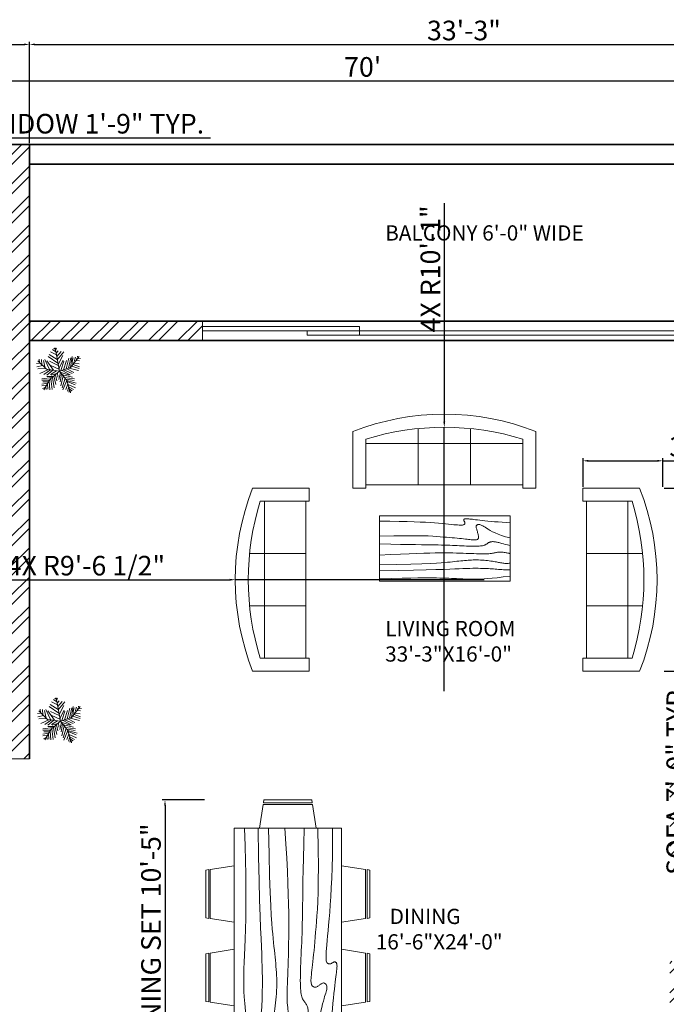
# Model space of a CAD drawing. Units: inches. Extents: x 416 to 1422, y 799 to 1634.
# Tile 3 of 5: x 746 to 1043, y 1174 to 1626. Entities that reach past the tile are written whole.
import ezdxf

# ---------------------------------------------------------------- set-up
doc = ezdxf.new("R2010")
doc.units = ezdxf.units.IN
doc.linetypes.add('ACAD_ISO02W100', pattern=[15, 12, -3])
for name, color, linetype, lineweight in [('A-ANNO-DIMS', 2, 'Continuous', 18), ('A-AREA-IDEN', 7, 'Continuous', 18), ('A-FURN', 8, 'Continuous', 18), ('A-GLAZ', 244, 'Continuous', 18), ('A-WALL', 7, 'Continuous', 35), ('A-WALL-HIDN', 7, 'ACAD_ISO02W100', 18), ('A-WALL-PATT', 252, 'Continuous', 13), ('L-PLNT', 3, 'Continuous', 13)]:
    doc.layers.add(name, color=color, linetype=linetype, lineweight=lineweight)
doc.styles.get("Standard").update_dxf_attribs({"font": 'arial.ttf'})
doc.dimstyles.new('ISO-25', dxfattribs={"dimtxt": 9, "dimasz": 2.5, "dimexe": 1.25, "dimexo": 0.625, "dimtad": 1, "dimlunit": 3, "dimtxsty": 'Standard', "dimcen": 2.5, "dimadec": 0, "dimazin": 0, "dimtfac": 1, "dimtmove": 0, "dimatfit": 3, "dimfxl": 1, "dimarcsym": 0})

# ---------------------------------------------------------------- blocks, each defined once
blk = doc.blocks.new('Dining Set - 36 x 72 in.')
for p, q in [((-22, 27.5), (-22.1562, 26.50042)), ((-5.8416, 26.5), (-22.1534, 26.5)), ((-22, 27.5), (-6, 27.5)), ((-5.8437, 26.49966), (-6, 27.5)), ((6, 27.5), (5.8438, 26.50042)), ((22.1584, 26.5), (5.8466, 26.5)), ((6, 27.5), (22, 27.5)), ((22.1563, 26.49966), (22, 27.5)), ((-22.2343, 26.00059), (-23.4847, 17.99762)), ((-22.2304, 26), (-5.7608, 26)), ((-4.5152, 17.99762), (-5.7655, 25.99926)), ((5.7657, 26.00059), (4.5153, 17.99762)), ((5.7696, 26), (22.2392, 26)), ((23.4848, 17.99762), (22.2345, 25.99926)), ((36, 18), (-36, 18)), ((-36, 18), (-36, -18)), ((36, -18), (36, 18)), ((-45.5, 8), (-44.5004, 8.15617)), ((-45.5, 8), (-45.5, -8)), ((-44.5, -8.15843), (-44.5, 8.15338)), ((-44.0006, 8.23428), (-35.9976, 9.48474)), ((-44, 8.23041), (-44, -8.23915)), ((44.0006, 8.23428), (35.9976, 9.48474)), ((44, 8.23041), (44, -8.23915)), ((44.5, -8.15843), (44.5, 8.15338)), ((45.5, 8), (44.5005, 8.15617)), ((45.5, 8), (45.5, -8)), ((-44.4997, -8.15631), (-45.5, -8)), ((-35.9976, -9.48476), (-43.9993, -8.2345)), ((35.9976, -9.48476), (43.9993, -8.2345)), ((44.4997, -8.15631), (45.5, -8)), ((-36, -18), (36, -18)), ((-22.2343, -26.0006), (-23.4847, -17.99762)), ((-4.5152, -17.99762), (-5.7655, -25.99928)), ((5.7657, -26.0006), (4.5153, -17.99762)), ((23.4848, -17.99762), (22.2345, -25.99928)), ((-22.2304, -26), (-5.7608, -26)), ((5.7696, -26), (22.2392, -26)), ((-22, -27.5), (-22.1562, -26.50044)), ((-5.8416, -26.5), (-22.1534, -26.5)), ((-22, -27.5), (-6, -27.5)), ((-5.8437, -26.49967), (-6, -27.5)), ((6, -27.5), (5.8438, -26.50044)), ((22.1584, -26.5), (5.8466, -26.5)), ((6, -27.5), (22, -27.5)), ((22.1563, -26.49967), (22, -27.5))]:
    blk.add_line(p, q)
for points in [[(-36, 15), (-31.1772, 14.97754), (-26.8079, 14.91406), (-22.8538, 14.81543), (-19.276, 14.6875), (-16.0362, 14.53613), (-13.0957, 14.36718), (-10.4159, 14.18652), (-7.9583, 14), (-5.6904, 13.81315), (-3.6035, 13.63021), (-1.6954, 13.45508), (0.0365, 13.29166), (1.5945, 13.14388), (2.9811, 13.01562), (4.1988, 12.9108), (5.25, 12.83333), (6.1393, 12.78613), (6.8802, 12.76823), (7.4883, 12.77767), (7.9792, 12.8125), (8.3685, 12.87077), (8.6719, 12.95052), (8.9049, 13.0498), (9.0833, 13.16666), (9.2205, 13.29899), (9.3216, 13.44401), (9.3895, 13.59879), (9.4271, 13.76041), (9.4373, 13.92594), (9.4232, 14.09245), (9.3875, 14.257), (9.3333, 14.41666), (9.2638, 14.56917), (9.1836, 14.71484), (9.0975, 14.85465), (9.0104, 14.98958), (8.9272, 15.1206), (8.8529, 15.2487), (8.7922, 15.37483), (8.75, 15.5), (8.7305, 15.62467), (8.7344, 15.74739), (8.7617, 15.86621), (8.8125, 15.97916), (8.8867, 16.08431), (8.9844, 16.17968), (9.1055, 16.26334), (9.25, 16.33333), (9.4189, 16.38802), (9.6172, 16.42708), (9.8506, 16.45052), (10.125, 16.45833), (10.4463, 16.45052), (10.8203, 16.42708), (11.2529, 16.38802), (11.75, 16.33333), (12.3184, 16.26318), (12.9694, 16.17838), (13.7151, 16.07991), (14.5677, 15.96875), (15.5395, 15.84586), (16.6426, 15.71224), (17.8893, 15.56884), (19.2917, 15.41666), (20.859, 15.25667), (22.5879, 15.08984), (24.4721, 14.91715), (26.5052, 14.73958), (28.6809, 14.5581), (30.9929, 14.3737), (33.4347, 14.18733), (36, 14)], [(-36, 10), (-28.9766, 10.14274), (-23.1725, 10.20442), (-18.4241, 10.19775), (-14.5677, 10.13541), (-11.4399, 10.03011), (-8.877, 9.89453), (-6.7154, 9.74137), (-4.7917, 9.58333), (-2.9698, 9.43082), (-1.2246, 9.28515), (0.4415, 9.14534), (2.026, 9.01041), (3.5266, 8.87939), (4.9408, 8.7513), (6.266, 8.62516), (7.5, 8.5), (8.6411, 8.37549), (9.6914, 8.2539), (10.6538, 8.13818), (11.5312, 8.03125), (12.3267, 7.93603), (13.043, 7.85547), (13.6831, 7.79248), (14.25, 7.75), (14.7471, 7.7303), (15.1797, 7.73307), (15.5537, 7.75732), (15.875, 7.80208), (16.1494, 7.86637), (16.3828, 7.94922), (16.5811, 8.04964), (16.75, 8.16666), (16.8944, 8.29915), (17.0143, 8.44531), (17.1089, 8.60319), (17.1771, 8.77083), (17.218, 8.94629), (17.2305, 9.1276), (17.2137, 9.31282), (17.1667, 9.5), (17.0895, 9.6875), (16.987, 9.875), (16.8649, 10.0625), (16.7292, 10.25), (16.5856, 10.4375), (16.4401, 10.625), (16.2985, 10.8125), (16.1667, 11), (16.05, 11.18733), (15.9518, 11.3737), (15.8752, 11.5581), (15.8229, 11.73958), (15.798, 11.91715), (15.8034, 12.08984), (15.842, 12.25667), (15.9167, 12.41666), (16.0295, 12.56836), (16.1784, 12.70833), (16.3605, 12.83268), (16.5729, 12.9375), (16.8127, 13.01888), (17.0768, 13.07291), (17.3625, 13.0957), (17.6667, 13.08333), (17.9894, 13.03312), (18.3418, 12.94726), (18.7382, 12.82918), (19.1927, 12.68229), (19.7195, 12.51001), (20.3327, 12.31575), (21.0465, 12.10294), (21.875, 11.875), (22.8357, 11.63354), (23.959, 11.37304), (25.2786, 11.08618), (26.8282, 10.76562), (28.6414, 10.40405), (30.752, 9.99414), (33.1936, 9.52856), (36, 9)], [(-36, 5.5), (-30.7157, 5.3348), (-26.069, 5.20963), (-21.9946, 5.11767), (-18.4271, 5.05208), (-15.3009, 5.00602), (-12.5508, 4.97265), (-10.1112, 4.94515), (-7.9167, 4.91666), (-5.909, 4.88167), (-4.0586, 4.83984), (-2.3429, 4.79215), (-0.7396, 4.73958), (0.7739, 4.6831), (2.22, 4.6237), (3.6213, 4.56233), (5, 4.5), (6.373, 4.43782), (7.7344, 4.3776), (9.0723, 4.32129), (10.375, 4.27083), (11.6309, 4.22819), (12.8281, 4.19531), (13.9551, 4.17415), (15, 4.16666), (15.954, 4.17448), (16.819, 4.19791), (17.6001, 4.23698), (18.3021, 4.29166), (18.9299, 4.36198), (19.4883, 4.44791), (19.9823, 4.54948), (20.4167, 4.66666), (20.7969, 4.79899), (21.1302, 4.94401), (21.4245, 5.09879), (21.6875, 5.26041), (21.9271, 5.42594), (22.1511, 5.59245), (22.3672, 5.757), (22.5834, 5.91666), (22.8065, 6.06868), (23.0404, 6.21093), (23.2879, 6.34147), (23.5521, 6.45833), (23.8358, 6.55957), (24.142, 6.64323), (24.4735, 6.70735), (24.8334, 6.75), (25.2235, 6.76969), (25.642, 6.76692), (26.0858, 6.74267), (26.5521, 6.69791), (27.0379, 6.63362), (27.5404, 6.55078), (28.0565, 6.45036), (28.5834, 6.33333), (29.1242, 6.19987), (29.7071, 6.04687), (30.3661, 5.87044), (31.1354, 5.66666), (32.0493, 5.43164), (33.142, 5.16146), (34.4475, 4.85221), (36, 4.5)], [(-36, -1), (-30.7915, -0.6591), (-26.0195, -0.38216), (-21.6519, -0.16284), (-17.6563, 0.00521), (-14.0005, 0.12833), (-10.6523, 0.21289), (-7.5796, 0.26522), (-4.75, 0.29166), (-2.134, 0.29793), (0.2878, 0.28711), (2.5317, 0.26163), (4.6146, 0.22396), (6.5529, 0.17651), (8.3633, 0.12174), (10.0623, 0.06209), (11.6667, 0), (13.1899, -0.06201), (14.6341, -0.1211), (15.9982, -0.17432), (17.2813, -0.21875), (18.4823, -0.25147), (19.6003, -0.26953), (20.6343, -0.27002), (21.5834, -0.25), (22.4481, -0.20768), (23.2357, -0.14584), (23.9549, -0.06836), (24.6146, 0.02083), (25.2235, 0.11784), (25.7904, 0.21875), (26.3241, 0.31966), (26.8334, 0.41666), (27.3265, 0.50618), (27.8099, 0.58593), (28.2894, 0.65397), (28.7709, 0.70833), (29.2601, 0.74707), (29.763, 0.76823), (30.2855, 0.76985), (30.8334, 0.75), (31.4088, 0.70784), (31.9994, 0.64713), (32.589, 0.57275), (33.1615, 0.48958), (33.7008, 0.4025), (34.1908, 0.3164), (34.6153, 0.23616), (34.9584, 0.16666), (35.2099, 0.11165), (35.3848, 0.07031), (35.504, 0.04069), (35.5886, 0.02083), (35.6594, 0.00879), (35.7377, 0.0026), (35.8442, 0.00032), (36, 0)], [(-36, -6.5), (-27.1843, -6.31267), (-20.084, -6.1263), (-14.469, -5.9419), (-10.1094, -5.76042), (-6.7752, -5.58285), (-4.2363, -5.41016), (-2.2629, -5.24333), (-0.625, -5.08334), (0.8708, -4.93099), (2.2715, -4.78646), (3.5872, -4.64974), (4.8281, -4.52084), (6.0046, -4.39974), (7.127, -4.28646), (8.2053, -4.18099), (9.25, -4.08334), (10.2705, -3.99382), (11.2734, -3.91407), (12.2647, -3.84603), (13.25, -3.79167), (14.2354, -3.75293), (15.2266, -3.73177), (16.2295, -3.73015), (17.25, -3.75), (18.2912, -3.79248), (19.3451, -3.85547), (20.4009, -3.93604), (21.4479, -4.03125), (22.4754, -4.13819), (23.4727, -4.25391), (24.4289, -4.37549), (25.3334, -4.5), (26.1785, -4.62492), (26.9694, -4.74935), (27.7145, -4.87281), (28.4219, -4.99479), (29.1, -5.11483), (29.7572, -5.23242), (30.4016, -5.34709), (31.0417, -5.45834), (31.6837, -5.56437), (32.3262, -5.65821), (32.9658, -5.73153), (33.599, -5.77604), (34.2224, -5.78345), (34.8327, -5.74545), (35.4264, -5.65373), (36, -5.5)], [(-36, -10), (-26.4022, -9.81299), (-18.4675, -9.62891), (-11.9839, -9.45069), (-6.7396, -9.28125), (-2.5226, -9.12354), (0.8789, -8.98047), (3.6769, -8.85498), (6.0833, -8.75), (8.2767, -8.66765), (10.3021, -8.60677), (12.1712, -8.56543), (13.8958, -8.54167), (15.4876, -8.53353), (16.9583, -8.53907), (18.3197, -8.55632), (19.5834, -8.58334), (20.7616, -8.61841), (21.8685, -8.66081), (22.9188, -8.71004), (23.9271, -8.76563), (24.9081, -8.82707), (25.8763, -8.89388), (26.8465, -8.96558), (27.8334, -9.04167), (28.8474, -9.12118), (29.8828, -9.20117), (30.93, -9.27824), (31.9792, -9.34896), (33.0205, -9.40991), (34.0443, -9.45768), (35.0407, -9.48885), (36, -9.5)], [(-36, -14.5), (-30.0881, -14.33513), (-25.0332, -14.21224), (-20.7312, -14.12647), (-17.0781, -14.07292), (-13.97, -14.04671), (-11.3027, -14.04297), (-8.9724, -14.05681), (-6.875, -14.08334), (-4.9224, -14.11833), (-3.0905, -14.16016), (-1.3709, -14.20785), (0.2448, -14.26042), (1.7647, -14.3169), (3.1973, -14.3763), (4.5507, -14.43767), (5.8333, -14.5), (7.0554, -14.5621), (8.235, -14.62175), (9.3922, -14.67652), (10.5469, -14.72396), (11.7192, -14.76164), (12.929, -14.78711), (14.1965, -14.79794), (15.5417, -14.79167), (16.9933, -14.76424), (18.6152, -14.70508), (20.4804, -14.60197), (22.6615, -14.44271), (25.2312, -14.21509), (28.2624, -13.9069), (31.8277, -13.50594), (36, -13)]]:
    blk.add_lwpolyline(points)
blk = doc.blocks.new('Table - Rectangular Woodgrain 60 x 30 in.')
for p, q in [((0, 0), (0, -30)), ((60, 0), (0, 0)), ((60, -30), (60, 0)), ((0, -30), (60, -30))]:
    blk.add_line(p, q)
for points in [[(0, -2.4), (4.8155, -2.418), (9.0302, -2.4688), (12.709, -2.5477), (15.9167, -2.65), (18.7181, -2.7711), (21.1781, -2.9063), (23.3616, -3.0508), (25.3333, -3.2), (27.1477, -3.3495), (28.8172, -3.4958), (30.3437, -3.636), (31.7291, -3.7667), (32.9756, -3.8849), (34.0849, -3.9875), (35.059, -4.0714), (35.9, -4.1334), (36.6114, -4.1711), (37.2041, -4.1854), (37.6906, -4.1779), (38.0833, -4.15), (38.3948, -4.1034), (38.6375, -4.0396), (38.8239, -3.9602), (38.9666, -3.8667), (39.0764, -3.7608), (39.1573, -3.6448), (39.2116, -3.521), (39.2416, -3.3917), (39.2498, -3.2593), (39.2385, -3.1261), (39.21, -2.9944), (39.1666, -2.8667), (39.111, -2.7447), (39.0468, -2.6281), (38.978, -2.5163), (38.9083, -2.4083), (38.8418, -2.3035), (38.7823, -2.201), (38.7337, -2.1001), (38.7, -2), (38.6844, -1.9003), (38.6875, -1.8021), (38.7094, -1.707), (38.75, -1.6167), (38.8094, -1.5326), (38.8875, -1.4563), (38.9844, -1.3893), (39.1, -1.3333), (39.2351, -1.2896), (39.3937, -1.2583), (39.5804, -1.2396), (39.8, -1.2333), (40.057, -1.2396), (40.3562, -1.2583), (40.7023, -1.2896), (41.1, -1.3333), (41.5547, -1.3895), (42.0755, -1.4573), (42.6721, -1.5361), (43.3542, -1.625), (44.1316, -1.7233), (45.014, -1.8302), (46.0114, -1.9449), (47.1333, -2.0667), (48.3862, -2.1947), (49.7625, -2.3281), (51.2513, -2.4663), (52.8416, -2.6083), (54.5226, -2.7535), (56.2833, -2.9011), (58.1127, -3.0501), (60, -3.2)], [(0, -9.2), (6.5759, -9.0858), (11.9385, -9.0365), (16.2527, -9.0418), (19.6833, -9.0917), (22.3952, -9.1759), (24.5531, -9.2844), (26.322, -9.4069), (27.8666, -9.5333), (29.3241, -9.6553), (30.7203, -9.7719), (32.0532, -9.8837), (33.3208, -9.9917), (34.5213, -10.0965), (35.6526, -10.199), (36.7128, -10.2999), (37.7, -10.4), (38.6129, -10.4996), (39.4531, -10.5969), (40.223, -10.6895), (40.925, -10.775), (41.5613, -10.8512), (42.1344, -10.9156), (42.6465, -10.966), (43.1, -11), (43.4976, -11.0158), (43.8437, -11.0136), (44.143, -10.9942), (44.4, -10.9583), (44.6195, -10.9069), (44.8062, -10.8406), (44.9648, -10.7603), (45.1, -10.6667), (45.2155, -10.5598), (45.3114, -10.4365), (45.3871, -10.2929), (45.4416, -10.125), (45.4743, -9.929), (45.4844, -9.7011), (45.4709, -9.4371), (45.4333, -9.1333), (45.3716, -8.7883), (45.2896, -8.4104), (45.1919, -8.0107), (45.0833, -7.6), (44.9685, -7.1893), (44.8521, -6.7896), (44.7388, -6.4117), (44.6333, -6.0667), (44.54, -5.7628), (44.4614, -5.4979), (44.4001, -5.2675), (44.3583, -5.0667), (44.3384, -4.8909), (44.3427, -4.7354), (44.3736, -4.5956), (44.4333, -4.4667), (44.5236, -4.3453), (44.6427, -4.2333), (44.7884, -4.1339), (44.9583, -4.05), (45.1501, -3.9849), (45.3614, -3.9417), (45.59, -3.9234), (45.8333, -3.9333), (46.0915, -3.9749), (46.3734, -4.0531), (46.6906, -4.1736), (47.0542, -4.3417), (47.4756, -4.5629), (47.9661, -4.8427), (48.5372, -5.1866), (49.2, -5.6), (49.9676, -6.0844), (50.8594, -6.625), (51.8965, -7.2031), (53.1, -7.8), (54.491, -8.3969), (56.0906, -8.975), (57.9199, -9.5156), (60, -10)], [(0, -12.8), (5.1847, -12.9322), (9.6213, -13.0323), (13.3963, -13.1059), (16.5958, -13.1583), (19.3063, -13.1952), (21.614, -13.2219), (23.6054, -13.2439), (25.3666, -13.2667), (26.9728, -13.2947), (28.4531, -13.3281), (29.8256, -13.3663), (31.1083, -13.4083), (32.3191, -13.4535), (33.476, -13.501), (34.597, -13.5501), (35.7, -13.6), (36.7984, -13.6497), (37.8875, -13.6979), (38.9578, -13.743), (40, -13.7833), (41.0047, -13.8174), (41.9625, -13.8438), (42.864, -13.8607), (43.7, -13.8667), (44.4631, -13.8604), (45.1552, -13.8417), (45.7801, -13.8104), (46.3416, -13.7667), (46.8439, -13.7104), (47.2906, -13.6417), (47.6858, -13.5604), (48.0333, -13.4667), (48.3375, -13.3608), (48.6042, -13.2448), (48.8396, -13.121), (49.05, -12.9917), (49.2417, -12.8593), (49.4208, -12.7261), (49.5937, -12.5944), (49.7667, -12.4667), (49.9452, -12.3451), (50.1323, -12.2313), (50.3303, -12.1268), (50.5416, -12.0333), (50.7686, -11.9524), (51.0135, -11.8854), (51.2788, -11.8341), (51.5666, -11.8), (51.8785, -11.7843), (52.2116, -11.7865), (52.562, -11.8059), (52.926, -11.8417), (53.2998, -11.8931), (53.6795, -11.9594), (54.0614, -12.0397), (54.4416, -12.1333), (54.8223, -12.2401), (55.2293, -12.3625), (55.6942, -12.5037), (56.2489, -12.6667), (56.9251, -12.8547), (57.7545, -13.0708), (58.7689, -13.3182), (60, -13.6)], [(0, -18), (5.124, -17.7273), (9.6609, -17.5057), (13.6705, -17.3303), (17.2125, -17.1958), (20.3467, -17.0973), (23.1328, -17.0297), (25.6307, -16.9878), (27.9, -16.9667), (29.9928, -16.9617), (31.9302, -16.9703), (33.7254, -16.9907), (35.3917, -17.0208), (36.9423, -17.0588), (38.3906, -17.1026), (39.7499, -17.1503), (41.0333, -17.2), (42.2519, -17.2496), (43.4073, -17.2969), (44.4986, -17.3395), (45.525, -17.375), (46.4858, -17.4012), (47.3802, -17.4156), (48.2074, -17.416), (48.9667, -17.4), (49.6583, -17.3662), (50.2872, -17.3167), (50.8595, -17.2547), (51.3812, -17.1833), (51.8584, -17.1057), (52.2971, -17.025), (52.7034, -16.9443), (53.0833, -16.8667), (53.443, -16.7951), (53.789, -16.7313), (54.128, -16.6768), (54.4666, -16.6334), (54.8115, -16.6024), (55.1693, -16.5854), (55.5465, -16.5841), (55.95, -16.6), (56.3828, -16.6337), (56.8346, -16.6823), (57.2915, -16.7418), (57.7396, -16.8084), (58.165, -16.878), (58.5539, -16.9469), (58.8924, -17.0111), (59.1666, -17.0667), (59.3679, -17.1107), (59.5078, -17.1438), (59.6032, -17.1675), (59.6708, -17.1833), (59.7275, -17.193), (59.7901, -17.1979), (59.8753, -17.1998), (60, -17.2)], [(0, -22.4), (8.0098, -22.2501), (14.4094, -22.1011), (19.4168, -21.9535), (23.25, -21.8083), (26.1269, -21.6663), (28.2656, -21.5281), (29.884, -21.3947), (31.2, -21.2667), (32.3967, -21.1448), (33.5172, -21.0292), (34.5697, -20.9198), (35.5625, -20.8167), (36.5037, -20.7198), (37.4015, -20.6292), (38.2642, -20.5448), (39.1, -20.4667), (39.9164, -20.3951), (40.7187, -20.3313), (41.5117, -20.2768), (42.3, -20.2333), (43.0883, -20.2024), (43.8812, -20.1854), (44.6836, -20.1841), (45.5, -20.2), (46.3328, -20.234), (47.1747, -20.2844), (48.0163, -20.3488), (48.8479, -20.425), (49.66, -20.5106), (50.4429, -20.6031), (51.1872, -20.7004), (51.8833, -20.8), (52.5246, -20.8999), (53.1166, -20.9995), (53.6681, -21.0983), (54.1875, -21.1958), (54.6834, -21.2919), (55.1646, -21.3859), (55.6394, -21.4777), (56.1167, -21.5667), (56.6028, -21.6515), (57.0961, -21.7266), (57.5929, -21.7852), (58.0896, -21.8208), (58.5823, -21.8268), (59.0674, -21.7964), (59.5412, -21.723), (60, -21.6)], [(0, -25.2), (8.6355, -25.0504), (15.7026, -24.9031), (21.4049, -24.7606), (25.9458, -24.625), (29.529, -24.4988), (32.3578, -24.3844), (34.6359, -24.284), (36.5667, -24.2), (38.3213, -24.1341), (39.9417, -24.0854), (41.437, -24.0523), (42.8167, -24.0333), (44.0901, -24.0268), (45.2667, -24.0313), (46.3557, -24.0451), (47.3667, -24.0667), (48.309, -24.0947), (49.1928, -24.1287), (50.0284, -24.168), (50.826, -24.2125), (51.5959, -24.2617), (52.3483, -24.3151), (53.0935, -24.3725), (53.8417, -24.4334), (54.6009, -24.497), (55.3699, -24.561), (56.1454, -24.6226), (56.9239, -24.6792), (57.7021, -24.7279), (58.4764, -24.7662), (59.2435, -24.7911), (60, -24.8)], [(0, -28.8), (5.6867, -28.6681), (10.45, -28.5698), (14.407, -28.5012), (17.675, -28.4584), (20.3711, -28.4374), (22.6125, -28.4344), (24.5164, -28.4455), (26.2, -28.4667), (27.762, -28.4947), (29.2276, -28.5281), (30.6033, -28.5663), (31.8958, -28.6084), (33.1118, -28.6535), (34.2578, -28.7011), (35.3405, -28.7501), (36.3666, -28.8), (37.3443, -28.8497), (38.288, -28.8974), (39.2137, -28.9412), (40.1375, -28.9792), (41.0753, -29.0093), (42.0432, -29.0297), (43.0572, -29.0384), (44.1333, -29.0333), (45.2936, -29.0114), (46.5843, -28.9641), (48.0579, -28.8816), (49.7666, -28.7542), (51.7629, -28.5721), (54.0989, -28.3255), (56.8272, -28.0048), (60, -27.6)]]:
    blk.add_lwpolyline(points)
blk = doc.blocks.new('Sofa - Roundback 7 ft.')
for p, q in [((-12.00002, -32.4421), (-12.00003, -6.5971)), ((11.99997, -32.4421), (11.99998, -6.5971)), ((-36.000027, -34), (-36.000027, -11.4696)), ((-35.999844, -13.3819), (35.9998, -13.3819)), ((35.99998, -34), (35.99998, -11.4696)), ((-36.000027, -32.4421), (35.99998, -32.4421))]:
    blk.add_line(p, q)
for points in [[(-36.000027, -34), (-42.000027, -34), (-42.000027, -8)], [(41.99998, -8), (41.99998, -34), (35.99998, -34)]]:
    blk.add_lwpolyline(points)
for centre, radius, start, end in [((0, -114.25), 114.25, 68.43141, 111.5686), ((-0.00001, -127.1968), 121.1968, 72.72033, 107.2797)]:
    blk.add_arc(centre, radius, start, end)
blk = doc.blocks.new('*U15')
for p, q in [((-8.737, 47.138), (-17.069, 52.711)), ((-10.186, 53.64), (-13.084, 55.962)), ((0, 0), (-10.5, 57)), ((-9.099, 51.782), (-6.563, 55.962)), ((-7.65, 43.423), (-2.578, 49.46)), ((-5.839, 35.992), (4.667, 48.067)), ((-31.5, 4.5), (-52.5, 25.5)), ((-48.585, 21.131), (-49.309, 29.026)), ((-43.513, 28.561), (-42.427, 15.558)), ((-38.442, 26.239), (-34.819, 7.663)), ((-35.544, 28.097), (-24.314, 3.947)), ((-14.533, 2.09), (-30.834, 25.31)), ((-3.665, 19.273), (-27.574, 35.527)), ((-5.114, 28.097), (-24.676, 40.636)), ((-7.288, 39.707), (-21.778, 46.673)), ((-5.114, 27.632), (10.463, 46.673)), ((-2.941, 16.486), (8.652, 37.85)), ((-1.129, 6.734), (9.014, 26.704)), ((3.942, 1.625), (11.187, 24.381)), ((10.101, 3.483), (17.708, 26.239)), ((16.259, 5.805), (23.142, 31.348)), ((22.055, 7.198), (27.489, 32.277)), ((27, 9), (48, 36)), ((27.127, 9.056), (31.112, 35.992)), ((31.836, 30.883), (32.561, 16.486)), ((35.096, 32.741), (37.27, 22.524)), ((38.719, 34.134), (41.979, 28.561)), ((40.53, 25.775), (48.862, 24.846)), ((43.791, 29.954), (51.036, 30.883)), ((44.153, 36.456), (45.239, 32.741)), ((-47.498, 19.737), (-55.83, 18.344)), ((-40.615, 13.7), (-55.105, 10.913)), ((-33.37, 6.269), (-52.207, 5.34)), ((-28.299, 3.483), (-47.86, -5.805)), ((-21.416, 3.018), (-38.079, -8.128)), ((0, 0), (-31.5, 4.5)), ((-15.982, 2.09), (-30.11, -9.521)), ((-24.314, 23.917), (-2.941, 13.7)), ((0, 0), (-22.5, -19.5)), ((-6.563, 1.161), (-21.416, -8.128)), ((-20.691, 13.7), (-1.129, 4.876)), ((0, 0), (27, 9)), ((0, 0), (18, -22.5)), ((6.478, 1.625), (26.04, -8.592)), ((11.187, 3.483), (30.749, -5.805)), ((18.07, 5.805), (35.096, -3.483)), ((24.229, 7.663), (46.688, 1.625)), ((29.662, 12.307), (48.137, 6.269)), ((33.285, 16.486), (48.862, 10.913)), ((36.183, 19.737), (48.137, 17.88)), ((-17.431, -15.094), (-42.789, -18.809)), ((-24.314, -21.596), (-42.427, -22.06)), ((-22.5, -19.5), (-37.5, -45)), ((-15.257, -12.772), (-30.11, -12.772)), ((-25.038, -23.918), (-22.865, -45.281)), ((-20.691, -18.345), (-17.793, -44.352)), ((-6.563, -5.805), (-19.967, -9.985)), ((-17.069, -15.094), (-12.721, -40.172)), ((-13.446, -11.378), (-8.737, -32.741)), ((-9.461, -8.592), (-6.201, -23.453)), ((-4.752, -3.483), (-3.665, -14.629)), ((2.493, -3.019), (-1.491, -20.202)), ((1.769, -2.555), (24.229, -9.521)), ((5.029, -6.27), (2.131, -25.775)), ((9.014, -11.378), (3.58, -35.992)), ((14.085, -16.951), (6.478, -40.172)), ((7.565, -9.056), (32.198, -14.629)), ((18.07, -22.524), (8.289, -45.745)), ((12.274, -15.094), (36.907, -18.809)), ((16.259, -19.738), (36.183, -22.989)), ((18, -22.5), (27, -52.5)), ((18.433, -22.524), (40.53, -29.026)), ((-28.299, -29.026), (-42.789, -31.348)), ((-30.834, -34.135), (-42.427, -35.528)), ((-34.457, -39.708), (-40.978, -42.494)), ((-26.849, -26.24), (-40.253, -25.775)), ((-32.646, -36.921), (-31.921, -44.352)), ((-29.023, -30.884), (-27.936, -43.887)), ((20.244, -30.419), (15.897, -44.816)), ((19.157, -25.311), (38.719, -33.206)), ((22.78, -37.85), (19.519, -48.532)), ((21.331, -32.741), (39.081, -40.636)), ((22.78, -38.314), (34.372, -44.816)), ((24.591, -45.745), (23.142, -50.854)), ((24.591, -43.423), (30.749, -47.603)), ((26.764, -49.925), (28.213, -50.854))]:
    blk.add_line(p, q)
blk = doc.blocks.new('*D17')
at = {"layer": 'A-ANNO-DIMS', "color": 0, "lineweight": -2, "transparency": 16777216}
for p, q in [((483.82, 1569.64), (483.82, 1599.55)), ((486.32, 1598.3), (1321.32, 1598.3)), ((1323.82, 1569.64), (1323.82, 1599.55))]:
    blk.add_line(p, q, dxfattribs=at)
at = {"layer": 'A-ANNO-DIMS', "color": 0, "transparency": 16777216}
for points in [[(486.32, 1598.72), (486.32, 1597.88), (483.82, 1598.3)], [(1321.32, 1598.72), (1321.32, 1597.88), (1323.82, 1598.3)]]:
    blk.add_solid(points, dxfattribs=at)
at = {"layer": 'Defpoints', "color": 0, "transparency": 16777216}
for p in [(1323.82, 1598.3), (483.82, 1569.01), (1323.82, 1569.01)]:
    blk.add_point(p, dxfattribs=at)
at = {"layer": 'A-ANNO-DIMS', "color": 0, "transparency": 16777216, "insert": (903.82, 1603.52), "char_height": 9, "attachment_point": 5}
blk.add_mtext("70'", dxfattribs=at)
blk = doc.blocks.new('*D25')
at = {"layer": 'A-ANNO-DIMS', "color": 0, "lineweight": -2, "transparency": 16777216}
for p, q in [((695.32, 1569.64), (695.32, 1573.41)), ((716.32, 1569.64), (716.32, 1573.41)), ((697.82, 1572.16), (713.82, 1572.16)), ((716.32, 1572.16), (833.96, 1572.16))]:
    blk.add_line(p, q, dxfattribs=at)
at = {"layer": 'A-ANNO-DIMS', "color": 0, "transparency": 16777216}
for points in [[(697.82, 1572.58), (697.82, 1571.75), (695.32, 1572.16)], [(713.82, 1572.58), (713.82, 1571.75), (716.32, 1572.16)]]:
    blk.add_solid(points, dxfattribs=at)
at = {"layer": 'Defpoints', "color": 0, "transparency": 16777216}
for p in [(695.32, 1569.01), (716.32, 1572.16), (716.32, 1569.01)]:
    blk.add_point(p, dxfattribs=at)
at = {"layer": 'A-ANNO-DIMS', "color": 0, "transparency": 16777216, "insert": (776.39, 1577.44), "char_height": 9, "attachment_point": 5}
blk.add_mtext('WINDOW 1\'-9" TYP.', dxfattribs=at)
blk = doc.blocks.new('*D27')
at = {"layer": 'A-ANNO-DIMS', "color": 0, "lineweight": -2, "transparency": 16777216}
for p, q in [((1042.27, 1411.23), (1055.49, 1411.23)), ((1054.24, 1408.73), (1054.24, 1329.73)), ((1042.27, 1327.23), (1055.49, 1327.23)), ((1054.24, 1327.23), (1054.24, 1230.94))]:
    blk.add_line(p, q, dxfattribs=at)
at = {"layer": 'A-ANNO-DIMS', "color": 0, "transparency": 16777216}
for points in [[(1053.83, 1408.73), (1054.66, 1408.73), (1054.24, 1411.23)], [(1053.83, 1329.73), (1054.66, 1329.73), (1054.24, 1327.23)]]:
    blk.add_solid(points, dxfattribs=at)
at = {"layer": 'Defpoints', "color": 0, "transparency": 16777216}
for p in [(1041.64, 1411.23), (1041.64, 1327.23), (1054.24, 1327.23)]:
    blk.add_point(p, dxfattribs=at)
at = {"layer": 'A-ANNO-DIMS', "color": 0, "transparency": 16777216, "insert": (1048.96, 1277.83), "char_height": 9, "attachment_point": 5, "rotation": 90}
blk.add_mtext('SOFA 7\'-0" TYP.', dxfattribs=at)
blk = doc.blocks.new('*D28')
at = {"layer": 'A-ANNO-DIMS', "color": 0, "lineweight": -2, "transparency": 16777216}
for p, q in [((1004.98, 1411.86), (1004.98, 1425.08)), ((1041.64, 1411.86), (1041.64, 1425.08)), ((1007.48, 1423.83), (1039.14, 1423.83)), ((1041.64, 1423.83), (1121.22, 1423.83))]:
    blk.add_line(p, q, dxfattribs=at)
at = {"layer": 'A-ANNO-DIMS', "color": 0, "transparency": 16777216}
for points in [[(1007.48, 1424.25), (1007.48, 1423.41), (1004.98, 1423.83)], [(1039.14, 1424.25), (1039.14, 1423.41), (1041.64, 1423.83)]]:
    blk.add_solid(points, dxfattribs=at)
at = {"layer": 'Defpoints', "color": 0, "transparency": 16777216}
for p in [(1041.64, 1423.83), (1004.98, 1411.23), (1041.64, 1411.23)]:
    blk.add_point(p, dxfattribs=at)
at = {"layer": 'A-ANNO-DIMS', "color": 0, "transparency": 16777216, "insert": (1082.68, 1429.11), "char_height": 9, "attachment_point": 5}
blk.add_mtext('3\'-0 1/2" TYP.', dxfattribs=at)
blk = doc.blocks.new('*D41')
at = {"layer": 'A-ANNO-DIMS', "color": 0, "lineweight": -2, "transparency": 16777216}
for p, q in [((831.14, 1268.11), (811.8, 1268.11)), ((813.05, 1265.61), (813.05, 1145.85)), ((831.14, 1143.35), (811.8, 1143.35))]:
    blk.add_line(p, q, dxfattribs=at)
at = {"layer": 'A-ANNO-DIMS', "color": 0, "transparency": 16777216}
for points in [[(812.63, 1265.61), (813.46, 1265.61), (813.05, 1268.11)], [(812.63, 1145.85), (813.46, 1145.85), (813.05, 1143.35)]]:
    blk.add_solid(points, dxfattribs=at)
at = {"layer": 'Defpoints', "color": 0, "transparency": 16777216}
for p in [(831.76, 1268.11), (813.05, 1143.35), (831.76, 1143.35)]:
    blk.add_point(p, dxfattribs=at)
at = {"layer": 'A-ANNO-DIMS', "color": 0, "transparency": 16777216, "insert": (807.77, 1205.73), "char_height": 9, "attachment_point": 5, "rotation": 90}
blk.add_mtext('DINING SET 10\'-5"', dxfattribs=at)
blk = doc.blocks.new('*D43')
at = {"layer": 'A-ANNO-DIMS', "color": 0, "lineweight": -2, "transparency": 16777216}
for p, q in [((483.19, 1569.01), (433, 1569.01)), ((434.25, 855.88), (434.25, 1566.51)), ((909.15, 853.38), (433, 853.38))]:
    blk.add_line(p, q, dxfattribs=at)
at = {"layer": 'A-ANNO-DIMS', "color": 0, "transparency": 16777216}
for points in [[(433.83, 1566.51), (434.67, 1566.51), (434.25, 1569.01)], [(433.83, 855.88), (434.67, 855.88), (434.25, 853.38)]]:
    blk.add_solid(points, dxfattribs=at)
at = {"layer": 'Defpoints', "color": 0, "transparency": 16777216}
for p in [(434.25, 1569.01), (483.82, 1569.01), (909.77, 853.38)]:
    blk.add_point(p, dxfattribs=at)
at = {"layer": 'A-ANNO-DIMS', "color": 0, "transparency": 16777216, "insert": (428.97, 1211.2), "char_height": 9, "attachment_point": 5, "rotation": 90}
blk.add_mtext('59\'-7 1/2"', dxfattribs=at)
blk = doc.blocks.new('*D51')
at = {"layer": 'A-ANNO-DIMS', "color": 0, "lineweight": -2, "transparency": 16777216}
for p, q in [((483.82, 1569.64), (483.82, 1616.26)), ((486.32, 1615.01), (748.32, 1615.01)), ((750.82, 1569.64), (750.82, 1616.26))]:
    blk.add_line(p, q, dxfattribs=at)
at = {"layer": 'A-ANNO-DIMS', "color": 0, "transparency": 16777216}
for points in [[(486.32, 1615.43), (486.32, 1614.6), (483.82, 1615.01)], [(748.32, 1615.43), (748.32, 1614.6), (750.82, 1615.01)]]:
    blk.add_solid(points, dxfattribs=at)
at = {"layer": 'Defpoints', "color": 0, "transparency": 16777216}
for p in [(750.82, 1615.01), (483.82, 1569.01), (750.82, 1569.01)]:
    blk.add_point(p, dxfattribs=at)
at = {"layer": 'A-ANNO-DIMS', "color": 0, "transparency": 16777216, "insert": (617.32, 1620.24), "char_height": 9, "attachment_point": 5}
blk.add_mtext('22\'-3"', dxfattribs=at)
blk = doc.blocks.new('*D52')
at = {"layer": 'A-ANNO-DIMS', "color": 0, "lineweight": -2, "transparency": 16777216}
for p, q in [((750.82, 1569.64), (750.82, 1616.26)), ((753.32, 1615.01), (1147.32, 1615.01)), ((1149.82, 1569.64), (1149.82, 1616.26))]:
    blk.add_line(p, q, dxfattribs=at)
at = {"layer": 'A-ANNO-DIMS', "color": 0, "transparency": 16777216}
for points in [[(753.32, 1615.43), (753.32, 1614.6), (750.82, 1615.01)], [(1147.32, 1615.43), (1147.32, 1614.6), (1149.82, 1615.01)]]:
    blk.add_solid(points, dxfattribs=at)
at = {"layer": 'Defpoints', "color": 0, "transparency": 16777216}
for p in [(1149.82, 1615.01), (750.82, 1569.01), (1149.82, 1569.01)]:
    blk.add_point(p, dxfattribs=at)
at = {"layer": 'A-ANNO-DIMS', "color": 0, "transparency": 16777216, "insert": (950.32, 1620.24), "char_height": 9, "attachment_point": 5}
blk.add_mtext('33\'-3"', dxfattribs=at)
blk = doc.blocks.new('*D58')
at = {"layer": 'A-ANNO-DIMS', "color": 0, "lineweight": -2, "transparency": 16777216}
for p, q in [((941.28, 1542.19), (941.28, 1441.73)), ((941.28, 1318.03), (941.28, 1439.23))]:
    blk.add_line(p, q, dxfattribs=at)
at = {"layer": 'A-ANNO-DIMS', "color": 0, "transparency": 16777216}
blk.add_solid([(940.87, 1441.73), (941.7, 1441.73), (941.28, 1439.23)], dxfattribs=at)
at = {"layer": 'Defpoints', "color": 0, "transparency": 16777216}
for p in [(941.28, 1439.23), (941.28, 1318.03)]:
    blk.add_point(p, dxfattribs=at)
at = {"layer": 'A-ANNO-DIMS', "color": 0, "transparency": 16777216, "insert": (936.06, 1511.95), "char_height": 9, "attachment_point": 5, "rotation": 90}
blk.add_mtext('4X R10\'-1"', dxfattribs=at)
blk = doc.blocks.new('*D59')
at = {"layer": 'A-ANNO-DIMS', "color": 0, "lineweight": -2, "transparency": 16777216}
for p, q in [((739.52, 1369.23), (842.8, 1369.23)), ((959.55, 1369.23), (845.3, 1369.23))]:
    blk.add_line(p, q, dxfattribs=at)
at = {"layer": 'A-ANNO-DIMS', "color": 0, "transparency": 16777216}
blk.add_solid([(842.8, 1369.65), (842.8, 1368.81), (845.3, 1369.23)], dxfattribs=at)
at = {"layer": 'Defpoints', "color": 0, "transparency": 16777216}
for p in [(845.3, 1369.23), (959.55, 1369.23)]:
    blk.add_point(p, dxfattribs=at)
at = {"layer": 'A-ANNO-DIMS', "color": 0, "transparency": 16777216, "insert": (776.75, 1374.51), "char_height": 9, "attachment_point": 5, "rotation": 359.9998}
blk.add_mtext('4X R9\'-6 1/2"', dxfattribs=at)

msp = doc.modelspace()

# ---------------------------------------------------------------- hatches: boundary and pattern name
at = {"layer": 'A-WALL-PATT'}
h = msp.add_hatch(dxfattribs=at)
h.set_pattern_fill('ANSI32', color=256)
h.paths.add_polyline_path([(695.32, 1569.013), (607.303, 1569.013), (607.303, 1560.013), (660.82, 1560.013), (660.82, 1419.013), (657.82, 1419.013), (657.82, 1413.013), (669.82, 1413.013), (669.82, 1446.013), (672.82, 1446.013), (672.82, 1452.013), (669.82, 1452.013), (669.82, 1560.013), (695.32, 1560.013)])
h.paths.add_polyline_path([(1323.82, 1311.283), (1314.82, 1311.283), (1314.82, 1287.013), (1242.82, 1287.013), (1242.82, 1383.013), (1245.82, 1383.013), (1245.82, 1392.013), (1236.82, 1392.013), (1236.82, 1339.513), (1158.82, 1339.513), (1158.82, 1431.013), (1149.82, 1431.013), (1149.82, 1287.013), (1044.82, 1287.013), (1044.82, 1242.013), (1053.82, 1242.013), (1053.82, 1278.013), (1221.82, 1278.013), (1221.82, 1233.013), (1230.82, 1233.013), (1230.82, 1278.013), (1314.82, 1278.013), (1314.82, 1225.894), (1323.82, 1225.894)])
h.paths.add_polyline_path([(1158.82, 1287.013), (1158.82, 1333.513), (1236.82, 1333.513), (1236.82, 1287.013)], flags=16)
h.paths.add_polyline_path([(1323.82, 1569.013), (1283.747, 1569.013), (1283.747, 1560.013), (1314.82, 1560.013), (1314.82, 1392.013), (1275.82, 1392.013), (1275.82, 1383.013), (1314.82, 1383.013), (1314.82, 1332.283), (1323.82, 1332.283)])
h.paths.add_polyline_path([(750.82, 1569.013), (716.32, 1569.013), (716.32, 1560.013), (741.82, 1560.013), (741.82, 1452.013), (702.82, 1452.013), (702.82, 1447.513), (702.82, 1446.013), (741.82, 1446.013), (741.82, 1287.013), (750.82, 1287.013)])
h.paths.add_polyline_path([(1158.82, 1560.013), (1223.747, 1560.013), (1223.747, 1569.013), (1149.82, 1569.013), (1149.82, 1467.013), (1158.82, 1467.013)])
h.paths.add_polyline_path([(1323.82, 1098.013), (1230.82, 1098.013), (1230.82, 1149.013), (1323.82, 1149.013), (1323.82, 1204.894), (1314.82, 1204.894), (1314.82, 1158.013), (1230.82, 1158.013), (1230.82, 1203.013), (1221.82, 1203.013), (1221.82, 1098.013), (1053.82, 1098.013), (1053.82, 1194.013), (1044.82, 1194.013), (1044.82, 1089.013), (1104.82, 1089.013), (1104.82, 1086.013), (1113.82, 1086.013), (1113.82, 1089.013), (1194.82, 1089.013), (1314.82, 1089.013), (1314.82, 897.013), (1194.82, 897.013), (1194.82, 1041.013), (1113.82, 1041.013), (1113.82, 1044.013), (1104.82, 1044.013), (1104.82, 1032.013), (1113.82, 1032.013), (1113.82, 1035.013), (1185.82, 1035.013), (1185.82, 969.013), (1113.82, 969.013), (1113.82, 1008.013), (1104.82, 1008.013), (1104.82, 969.013), (1088.452, 969.013), (1088.452, 960.013), (1185.82, 960.013), (1185.82, 888.013), (1323.82, 888.013)])
h = msp.add_hatch(dxfattribs=at)
h.set_pattern_fill('ANSI32', color=256)
h.paths.add_polyline_path([(830.32, 1488.013), (750.82, 1488.013), (750.82, 1479.013), (830.32, 1479.013)])
h.paths.add_polyline_path([(1149.82, 1488.013), (1070.32, 1488.013), (1070.32, 1479.013), (1149.82, 1479.013)])

# ---------------------------------------------------------------- linework, layer by layer
at = {"layer": 'A-GLAZ'}
for p, q in [((830.32, 1479.013), (830.32, 1488.013)), ((830.32, 1485.513), (902.32, 1485.513)), ((830.32, 1483.513), (1070.32, 1483.513)), ((878.32, 1481.513), (878.32, 1483.513)), ((902.32, 1481.513), (902.32, 1485.513)), ((878.32, 1481.513), (1070.32, 1481.513))]:
    msp.add_line(p, q, dxfattribs=at)
at = {"layer": 'A-WALL'}
for p, q in [((483.82, 1569.013), (1323.82, 1569.013)), ((750.82, 1569.013), (750.82, 1287.013)), ((750.82, 1560.013), (1149.82, 1560.013)), ((750.82, 1488.013), (1149.82, 1488.013)), ((750.82, 1479.013), (1149.82, 1479.013))]:
    msp.add_line(p, q, dxfattribs=at)
at = {"layer": 'A-WALL-HIDN'}
msp.add_line((750.82, 1287.013), (741.82, 1287.013), dxfattribs=at)

# ---------------------------------------------------------------- block references
at = {"layer": 'A-FURN'}
for name, p in [('Sofa - Roundback 7 ft.', (941.284, 1445.231)), ('Table - Rectangular Woodgrain 60 x 30 in.', (911.519, 1398.492))]:
    msp.add_blockref(name, p, dxfattribs=at)
for p, rotation in [((845.296, 1369.231), 90), ((1038.976, 1369.231), 270)]:
    msp.add_blockref('Sofa - Roundback 7 ft.', p, dxfattribs=dict(at, rotation=rotation))
at = {"layer": 'A-FURN', "xscale": 1.371038100763723, "yscale": 1.371038100763723, "zscale": 1.371038100763723, "rotation": 270.0000000000002}
msp.add_blockref('Dining Set - 36 x 72 in.', (869.465, 1205.728), dxfattribs=at)
at = {"layer": 'L-PLNT', "xscale": 0.1889003163570017, "yscale": 0.1889003163570017, "zscale": 0.1889003163570017}
for p in [(764.537, 1464.989), (764.996, 1304.273)]:
    msp.add_blockref('*U15', p, dxfattribs=at)

# ---------------------------------------------------------------- texts
at = {"layer": 'A-AREA-IDEN', "char_height": 7, "attachment_point": 1}
for s, width, insert in [('BALCONY 6\'-0" WIDE', 108.72462, (914.134, 1531.958)), ('LIVING ROOM \\P33\'-3"X16\'-0"', 64.41546, (914.134, 1350.301)), ('   DINING         16\'-6"X24\'-0"', 55.68891, (909.802, 1218.124))]:
    msp.add_mtext_dynamic_manual_height_columns(s, width=width, gutter_width=12.5, heights=[0], dxfattribs=dict(at, insert=insert))

# ---------------------------------------------------------------- dimensions: what is measured, and where the dimension line sits
at = {"layer": 'A-ANNO-DIMS'}
for base, p1, p2, override, picture, middle in [((750.82, 1615.013), (483.82, 1569.013), (750.82, 1569.013), {"dimdec": 1, "dimlfac": 1, "dimrnd": 0, "dimzin": 1, "dimdsep": 46, "dimlunit": 4, "dimfrac": 2}, '*D51', (617.32, 1620.236)), ((1149.82, 1615.013), (750.82, 1569.013), (1149.82, 1569.013), {"dimdec": 1, "dimlfac": 1, "dimrnd": 0, "dimzin": 1, "dimdsep": 46, "dimlunit": 4, "dimfrac": 2}, '*D52', (950.32, 1620.236)), ((1323.82, 1598.301), (483.82, 1569.013), (1323.82, 1569.013), {"dimclrd": 0, "dimclre": 0, "dimclrt": 0}, '*D17', (903.82, 1603.522))]:
    dim = msp.add_linear_dim(base=base, p1=p1, p2=p2, dimstyle='ISO-25', override=override, dxfattribs=at)
    dim.commit()
    dim.dimension.update_dxf_attribs({"geometry": picture, "text_midpoint": middle})
for base, p1, p2, text, picture, middle in [((716.32, 1572.163), (695.32, 1569.013), (716.32, 1569.013), 'WINDOW <> TYP.', '*D25', (776.389, 1577.444)), ((1041.643, 1423.831), (1004.976, 1411.231), (1041.643, 1411.231), '<> TYP.', '*D28', (1082.68, 1429.112))]:
    dim = msp.add_linear_dim(base=base, p1=p1, p2=p2, text=text, dimstyle='ISO-25', override={"dimdec": 1, "dimlfac": 1, "dimrnd": 0, "dimzin": 1, "dimdsep": 46, "dimlunit": 4, "dimfrac": 2}, dxfattribs=at)
    dim.commit()
    dim.dimension.update_dxf_attribs({"geometry": picture, "text_midpoint": middle})
dim = msp.add_linear_dim(base=(434.249, 1569.013), p1=(909.773, 853.38), p2=(483.82, 1569.013), angle=90, dimstyle='ISO-25', override={"dimdec": 1, "dimlfac": 1, "dimrnd": 0, "dimzin": 1, "dimdsep": 46, "dimlunit": 4, "dimfrac": 2}, dxfattribs=at)
dim.commit()
dim.dimension.update_dxf_attribs({"geometry": '*D43', "text_midpoint": (428.97, 1211.196)})
for center, mpoint, picture, middle in [((941.284, 1318.034), (941.284, 1439.231), '*D58', (941.284, 1511.949)), ((959.546124, 1369.230665), (845.296124, 1369.231), '*D59', (776.746124, 1369.231201))]:
    dim = msp.add_radius_dim(center=center, mpoint=mpoint, text='4X <>', dimstyle='ISO-25', override={"dimdec": 1, "dimlfac": 1, "dimrnd": 0, "dimzin": 1, "dimdsep": 46, "dimlunit": 4, "dimfrac": 2}, dxfattribs=at)
    dim.commit()
    dim.dimension.update_dxf_attribs({"geometry": picture, "text_midpoint": middle, "dimtype": 164})
for base, p1, p2, text, picture, middle in [((1054.243, 1327.231), (1041.643, 1411.231), (1041.643, 1327.231), 'SOFA <> TYP.', '*D27', (1048.961, 1277.835)), ((813.047, 1143.346), (831.761, 1268.11), (831.761, 1143.346), 'DINING SET <>', '*D41', (807.768, 1205.728))]:
    dim = msp.add_linear_dim(base=base, p1=p1, p2=p2, angle=270, text=text, dimstyle='ISO-25', override={"dimdec": 1, "dimlfac": 1, "dimrnd": 0, "dimzin": 1, "dimdsep": 46, "dimlunit": 4, "dimfrac": 2}, dxfattribs=at)
    dim.commit()
    dim.dimension.update_dxf_attribs({"geometry": picture, "text_midpoint": middle})

doc.saveas('drawing.dxf')
